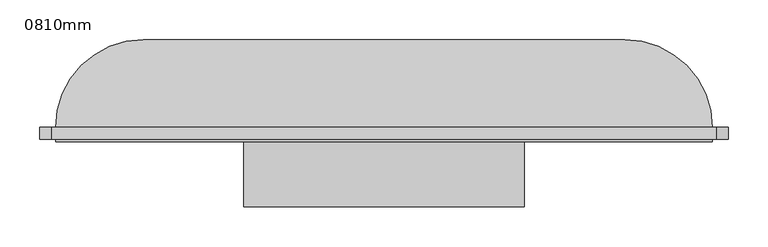
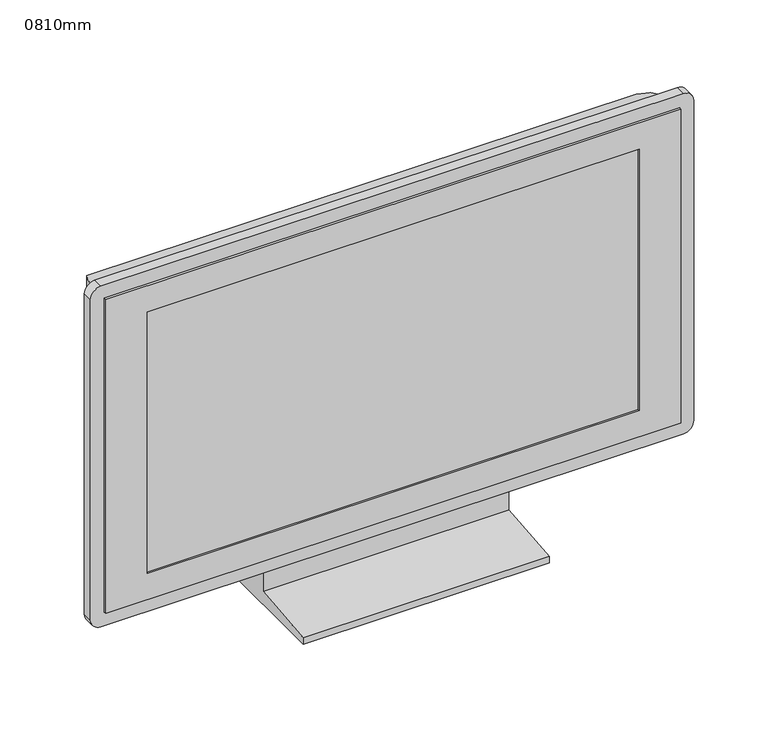
"""IFC4 building model written with IfcOpenShell, lengths in millimetres: furniture geometry, 0810mm."""

from ifc_helpers import new_model, si_unit, point, frame, frame_2d, origin, place, context, project, spatial, polyline, circle_curve, ellipse_curve, trimmed, segment, composite_curve, outline, extrude, faceted_brep, source, transform, mapped, element, save
from ifc_brep_helpers import plane_surface, cylinder_surface, advanced_brep


def furniture_0810mm_56245f3a(model_context):
    return source(origin(), model_context, "Body", "SolidModel", [
        extrude(outline(polyline([(-51.4613764, 80.0), (-1.4613764, 80.0), (48.5386236, 0.0), (-151.4613764, 0.0), (-151.4613764, 10.0), (-51.4613764, 20.0), (-51.4613764, 80.0)])), frame((-180.4346678, 0.0, 0.0), z_axis=(1.0, 0.0, 0.0), x_axis=(0.0, 1.0, 0.0)), (0.0, 0.0, 1.0), 352.9803073),
        faceted_brep([(409.0357931, -69.4613764, 557.1392838), (-416.9248214, -69.4613764, 557.1392838), (-416.9248214, -69.4613764, 80.0), (409.0357931, -69.4613764, 80.0), (-356.9248214, -69.4613764, 517.1392838), (349.0357931, -69.4613764, 517.1392838), (349.0357931, -69.4613764, 120.0), (-356.9248214, -69.4613764, 120.0), (409.0357931, -51.4613764, 557.1392838), (409.0357931, -51.4613764, 80.0), (-416.9248214, -51.4613764, 80.0), (-416.9248214, -51.4613764, 557.1392838), (-356.9248214, -66.4613764, 517.1392838), (-356.9248214, -66.4613764, 120.0), (349.0357931, -66.4613764, 120.0), (349.0357931, -66.4613764, 517.1392838)], [[[0, 1, 2, 3], [4, 5, 6, 7]], [[8, 9, 10, 11]], [[1, 0, 8, 11]], [[2, 1, 11, 10]], [[3, 2, 10, 9]], [[0, 3, 9, 8]], [[12, 13, 14, 15]], [[12, 15, 5, 4]], [[15, 14, 6, 5]], [[14, 13, 7, 6]], [[13, 12, 4, 7]]]),
        extrude(outline(composite_curve([segment(polyline([(577.1392838, 414.0357931), (577.1392838, -421.9248214)]), True, "CONTINUOUS"), segment(trimmed(circle_curve(frame_2d((562.1392838, -421.9248214)), 15.0), [point((577.1392838, -421.9248214))], [point((562.1392838, -436.9248214))], False, "CARTESIAN"), True, "CONTINUOUS"), segment(polyline([(562.1392838, -436.9248214), (75.0, -436.9248214)]), True, "CONTINUOUS"), segment(trimmed(circle_curve(frame_2d((75.0, -421.9248214)), 15.0), [point((75.0, -436.9248214))], [point((60.0, -421.9248214))], False, "CARTESIAN"), True, "CONTINUOUS"), segment(polyline([(60.0, -421.9248214), (60.0, 414.0357931)]), True, "CONTINUOUS"), segment(trimmed(circle_curve(frame_2d((75.0, 414.0357931)), 15.0), [point((60.0, 414.0357931))], [point((75.0, 429.0357931))], False, "CARTESIAN"), True, "CONTINUOUS"), segment(polyline([(75.0, 429.0357931), (562.1392838, 429.0357931)]), True, "CONTINUOUS"), segment(trimmed(circle_curve(frame_2d((562.1392838, 414.0357931)), 15.0), [point((562.1392838, 429.0357931))], [point((577.1392838, 414.0357931))], False, "CARTESIAN"), True, "CONTINUOUS")], self_intersect=False), holes=[polyline([(557.1392838, 409.0357931), (80.0, 409.0357931), (80.0, -416.9248214), (557.1392838, -416.9248214), (557.1392838, 409.0357931)])]), frame((0.0, -66.4613764, 0.0), z_axis=(0.0, 1.0, 0.0), x_axis=(0.0, 0.0, 1.0)), (0.0, 0.0, 1.0), 15.0),
        advanced_brep(
        [(-416.9248214, -51.4613764, 80.0), (409.0357931, -51.4613764, 80.0), (409.0357931, -51.4613764, 557.1392838), (-416.9248214, -51.4613764, 557.1392838), (299.0357931, 58.5386236, 80.0), (-306.9248214, 58.5386236, 80.0), (-306.9248214, 58.5386236, 447.1392838), (299.0357931, 58.5386236, 447.1392838)],
        [
            (0, 1),
            (1, 2),
            (2, 3),
            (3, 0),
            (4, 5),
            (5, 6),
            (6, 7),
            (7, 4),
            (0, 5, circle_curve(frame((-306.9248214, -51.4613764, 80.0), z_axis=(0.0, 0.0, -1.0), x_axis=(-1.0, 0.0, 0.0)), 110.0)),
            (4, 1, circle_curve(frame((299.0357931, -51.4613764, 80.0), z_axis=(0.0, 0.0, -1.0), x_axis=(1.0, 0.0, 0.0)), 110.0)),
            (7, 2, ellipse_curve(frame((299.0357931, -51.4613764, 447.1392838), z_axis=(0.7071067811865475, 0.0, -0.7071067811865475), x_axis=(0.7071067811865474, 0.0, 0.7071067811865476)), 155.5634919, 110.0)),
            (6, 3, ellipse_curve(frame((-306.9248214, -51.4613764, 447.1392838), z_axis=(0.7071067811865475, 0.0, 0.7071067811865475), x_axis=(-0.7071067811865476, 0.0, 0.7071067811865474)), 155.5634919, 110.0)),
        ],
        [
            plane_surface(frame((-416.9248214, -51.4613764, 557.1392838), z_axis=(0.0, -1.0, 0.0), x_axis=(-1.0, 0.0, 0.0))),
            plane_surface(frame((-416.9248214, 58.5386236, 557.1392838), z_axis=(0.0, 1.0, 0.0), x_axis=(1.0, 0.0, 0.0))),
            plane_surface(frame((-416.9248214, -51.4613764, 80.0), z_axis=(0.0, 0.0, -1.0), x_axis=(0.0, 1.0, 0.0))),
            cylinder_surface(frame((299.0357931, -51.4613764, 80.0), z_axis=(0.0, 0.0, 1.0), x_axis=(1.0, 0.0, 0.0)), 110.0),
            cylinder_surface(frame((409.0357931, -51.4613764, 447.1392838), z_axis=(-1.0, 0.0, 0.0), x_axis=(0.0, 0.0, 1.0)), 110.0),
            cylinder_surface(frame((-306.9248214, -51.4613764, 557.1392838), z_axis=(0.0, 0.0, -1.0), x_axis=(-1.0, 0.0, 0.0)), 110.0),
        ],
        [
            (0, [[1, 2, 3, 4]]),
            (1, [[5, 6, 7, 8]]),
            (2, [[-1, 9, -5, 10]]),
            (3, [[11, -2, -10, -8]]),
            (4, [[-11, -7, 12, -3]]),
            (5, [[-12, -6, -9, -4]]),
        ],
    ),
    ])


if __name__ == "__main__":
    model = new_model("IFC4")
    model_context = context("Model", 3, world=origin())
    ifc_project = project(units=[si_unit("LENGTHUNIT", "METRE", prefix="MILLI")], contexts=[model_context])
    site = spatial("IfcSite", under=ifc_project)
    building = spatial("IfcBuilding", under=site)
    placement = place(None, origin())
    furniture_0810mm_shape = furniture_0810mm_56245f3a(model_context)
    element("IfcFurniture", 1, ObjectType="0810mm", at=placement, inside=building, context=model_context, shape_type="MappedRepresentation", body=[
        mapped(furniture_0810mm_shape, transform((0.0, 0.0, 0.0), x_axis=(1.0, 0.0, 0.0), y_axis=(0.0, 1.0, 0.0), z_axis=(0.0, 0.0, 1.0))),
    ])
    save(model, "model.ifc")

# Revit data of these elements
# Type "0810mm"
#   SinAng = 0' - 0.0193"
#   L = 2' - 3.79372"
#   H = 1' - 3.6354"
#   Thickness = 0' - 4.33071"
#   Diagonal = 2' - 7.88976"
#   CosAng = 0' - 0.03431"
#   Stand [instance default] = yes
#   Default Elevation = 0
# Element 1 (IfcFurniture, "0810mm")
#   Materials on its faces: "TV - Black", "TV - Glass", "TV - Screen"
# Materials
#   "TV - Black": colour RGB 49 49 49, transparency 0
#   "TV - Glass": colour RGB 157 157 157, transparency 0.9
#   "TV - Screen": colour RGB 0 0 0, transparency 0
